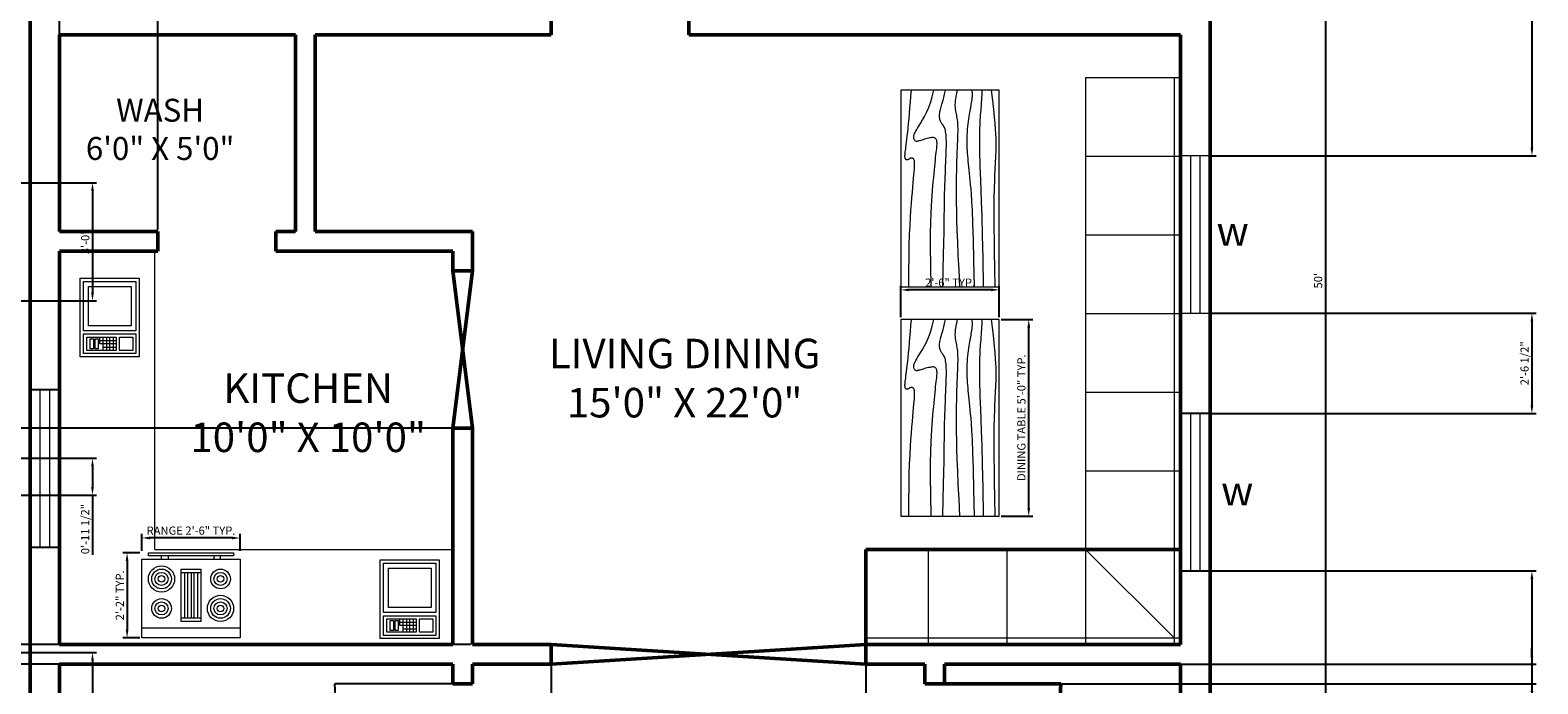
# Model space of a CAD drawing. Units: inches. Extents: x 3688 to 4628, y 1593 to 2337.
# Tile 6 of 7: x 4168 to 4628, y 1872 to 2072. Entities that reach past the tile are written whole.
import ezdxf

# ---------------------------------------------------------------- set-up
doc = ezdxf.new("R2010")
doc.units = ezdxf.units.IN
for name, color, linetype, lineweight in [('A-ANNO-DIMS', 2, 'Continuous', 18), ('A-ANNO-TEXT', 7, 'Continuous', 18), ('A-AREA-IDEN', 7, 'Continuous', 25), ('A-DOOR', 4, 'Continuous', 25), ('A-EQPM', 8, 'Continuous', 18), ('A-FLOR-FIXT', 8, 'Continuous', 18), ('A-FURN', 8, 'Continuous', 18), ('A-GLAZ', 4, 'Continuous', 25), ('A-WALL', 7, 'Continuous', 50)]:
    doc.layers.add(name, color=color, linetype=linetype, lineweight=lineweight)
doc.styles.get("Standard").update_dxf_attribs({"font": 'arial.ttf'})
doc.dimstyles.new('ISO-25', dxfattribs={"dimtxt": 2.5, "dimasz": 2.5, "dimexe": 1.25, "dimexo": 0.625, "dimtad": 1, "dimdec": 0, "dimlunit": 3, "dimtxsty": 'Standard', "dimcen": 2.5, "dimadec": 0, "dimazin": 0, "dimtfac": 1, "dimtdec": 0, "dimtmove": 0, "dimatfit": 3, "dimfxl": 1, "dimarcsym": 0})

# ---------------------------------------------------------------- blocks, each defined once
blk = doc.blocks.new('Microwave')
for p, q in [((18, 10), (22, 10)), ((19, 7), (19, 11)), ((20, 11), (20, 7)), ((21, 7), (21, 11)), ((22, 9), (18, 9)), ((18, 8), (22, 8)), ((22, 7), (18, 7)), ((20, 6), (18, 6)), ((19, 6), (19, 7)), ((20, 7), (20, 6))]:
    blk.add_line(p, q)
for points in [[(0, 0), (0, 18), (24, 18), (24, 0)], [(1, 1), (1, 17), (16, 17), (16, 1)], [(2.5, 2.5), (2.5, 15.5), (14.5, 15.5), (14.5, 2.5)], [(17, 1), (17, 17), (23, 17), (23, 1)], [(18, 12), (18, 16), (22, 16), (22, 12)], [(18, 2), (18, 11), (22, 11), (22, 2)], [(18.5, 4.5), (18.5, 5.5), (21.5, 5.5), (21.5, 4.5)], [(18.5, 3), (18.5, 4), (21.5, 4), (21.5, 3)]]:
    blk.add_lwpolyline(points, close=True)
blk = doc.blocks.new('Range-Oven - 30 in top')
for p, q in [((0, -3), (30, -3)), ((12, -6), (18, -6)), ((13, -20), (13, -6)), ((14, -6), (14, -20)), ((15, -20), (15, -6)), ((16, -6), (16, -20)), ((17, -20), (17, -6)), ((18, -20), (12, -20)), ((6, -24), (6, -25)), ((8, -25), (8, -24)), ((22, -25), (22, -24)), ((24, -24), (24, -25))]:
    blk.add_line(p, q)
for points in [[(0, -24), (0, 0), (30, 0), (30, -24)], [(12, -21), (12, -5), (18, -5), (18, -21)], [(2, -26), (2, -25), (28, -25), (28, -26)]]:
    blk.add_lwpolyline(points, close=True)
for centre, radius in [((6, -9), 4), ((6, -9), 3), ((6, -9), 2), ((6, -9), 1), ((24, -9), 3), ((24, -9), 2), ((24, -9), 1), ((6, -18), 3), ((6, -18), 2), ((6, -18), 1), ((24, -18), 4), ((24, -18), 3), ((24, -18), 2), ((24, -18), 1)]:
    blk.add_circle(centre, radius)
blk = doc.blocks.new('Table - Rectangular Woodgrain 60 x 30 in.')
for p, q in [((0, 0), (0, -30)), ((60, 0), (0, 0)), ((60, -30), (60, 0)), ((0, -30), (60, -30))]:
    blk.add_line(p, q)
for points in [[(0, -2.4), (4.8155, -2.418), (9.0302, -2.4688), (12.709, -2.5477), (15.9167, -2.65), (18.7181, -2.7711), (21.1781, -2.9063), (23.3616, -3.0508), (25.3333, -3.2), (27.1477, -3.3495), (28.8172, -3.4958), (30.3437, -3.636), (31.7291, -3.7667), (32.9756, -3.8849), (34.0849, -3.9875), (35.059, -4.0714), (35.9, -4.1334), (36.6114, -4.1711), (37.2041, -4.1854), (37.6906, -4.1779), (38.0833, -4.15), (38.3948, -4.1034), (38.6375, -4.0396), (38.8239, -3.9602), (38.9666, -3.8667), (39.0764, -3.7608), (39.1573, -3.6448), (39.2116, -3.521), (39.2416, -3.3917), (39.2498, -3.2593), (39.2385, -3.1261), (39.21, -2.9944), (39.1666, -2.8667), (39.111, -2.7447), (39.0468, -2.6281), (38.978, -2.5163), (38.9083, -2.4083), (38.8418, -2.3035), (38.7823, -2.201), (38.7337, -2.1001), (38.7, -2), (38.6844, -1.9003), (38.6875, -1.8021), (38.7094, -1.707), (38.75, -1.6167), (38.8094, -1.5326), (38.8875, -1.4563), (38.9844, -1.3893), (39.1, -1.3333), (39.2351, -1.2896), (39.3937, -1.2583), (39.5804, -1.2396), (39.8, -1.2333), (40.057, -1.2396), (40.3562, -1.2583), (40.7023, -1.2896), (41.1, -1.3333), (41.5547, -1.3895), (42.0755, -1.4573), (42.6721, -1.5361), (43.3542, -1.625), (44.1316, -1.7233), (45.014, -1.8302), (46.0114, -1.9449), (47.1333, -2.0667), (48.3862, -2.1947), (49.7625, -2.3281), (51.2513, -2.4663), (52.8416, -2.6083), (54.5226, -2.7535), (56.2833, -2.9011), (58.1127, -3.0501), (60, -3.2)], [(0, -9.2), (6.5759, -9.0858), (11.9385, -9.0365), (16.2527, -9.0418), (19.6833, -9.0917), (22.3952, -9.1759), (24.5531, -9.2844), (26.322, -9.4069), (27.8666, -9.5333), (29.3241, -9.6553), (30.7203, -9.7719), (32.0532, -9.8837), (33.3208, -9.9917), (34.5213, -10.0965), (35.6526, -10.199), (36.7128, -10.2999), (37.7, -10.4), (38.6129, -10.4996), (39.4531, -10.5969), (40.223, -10.6895), (40.925, -10.775), (41.5613, -10.8512), (42.1344, -10.9156), (42.6465, -10.966), (43.1, -11), (43.4976, -11.0158), (43.8437, -11.0136), (44.143, -10.9942), (44.4, -10.9583), (44.6195, -10.9069), (44.8062, -10.8406), (44.9648, -10.7603), (45.1, -10.6667), (45.2155, -10.5598), (45.3114, -10.4365), (45.3871, -10.2929), (45.4416, -10.125), (45.4743, -9.929), (45.4844, -9.7011), (45.4709, -9.4371), (45.4333, -9.1333), (45.3716, -8.7883), (45.2896, -8.4104), (45.1919, -8.0107), (45.0833, -7.6), (44.9685, -7.1893), (44.8521, -6.7896), (44.7388, -6.4117), (44.6333, -6.0667), (44.54, -5.7628), (44.4614, -5.4979), (44.4001, -5.2675), (44.3583, -5.0667), (44.3384, -4.8909), (44.3427, -4.7354), (44.3736, -4.5956), (44.4333, -4.4667), (44.5236, -4.3453), (44.6427, -4.2333), (44.7884, -4.1339), (44.9583, -4.05), (45.1501, -3.9849), (45.3614, -3.9417), (45.59, -3.9234), (45.8333, -3.9333), (46.0915, -3.9749), (46.3734, -4.0531), (46.6906, -4.1736), (47.0542, -4.3417), (47.4756, -4.5629), (47.9661, -4.8427), (48.5372, -5.1866), (49.2, -5.6), (49.9676, -6.0844), (50.8594, -6.625), (51.8965, -7.2031), (53.1, -7.8), (54.491, -8.3969), (56.0906, -8.975), (57.9199, -9.5156), (60, -10)], [(0, -12.8), (5.1847, -12.9322), (9.6213, -13.0323), (13.3963, -13.1059), (16.5958, -13.1583), (19.3063, -13.1952), (21.614, -13.2219), (23.6054, -13.2439), (25.3666, -13.2667), (26.9728, -13.2947), (28.4531, -13.3281), (29.8256, -13.3663), (31.1083, -13.4083), (32.3191, -13.4535), (33.476, -13.501), (34.597, -13.5501), (35.7, -13.6), (36.7984, -13.6497), (37.8875, -13.6979), (38.9578, -13.743), (40, -13.7833), (41.0047, -13.8174), (41.9625, -13.8438), (42.864, -13.8607), (43.7, -13.8667), (44.4631, -13.8604), (45.1552, -13.8417), (45.7801, -13.8104), (46.3416, -13.7667), (46.8439, -13.7104), (47.2906, -13.6417), (47.6858, -13.5604), (48.0333, -13.4667), (48.3375, -13.3608), (48.6042, -13.2448), (48.8396, -13.121), (49.05, -12.9917), (49.2417, -12.8593), (49.4208, -12.7261), (49.5937, -12.5944), (49.7667, -12.4667), (49.9452, -12.3451), (50.1323, -12.2313), (50.3303, -12.1268), (50.5416, -12.0333), (50.7686, -11.9524), (51.0135, -11.8854), (51.2788, -11.8341), (51.5666, -11.8), (51.8785, -11.7843), (52.2116, -11.7865), (52.562, -11.8059), (52.926, -11.8417), (53.2998, -11.8931), (53.6795, -11.9594), (54.0614, -12.0397), (54.4416, -12.1333), (54.8223, -12.2401), (55.2293, -12.3625), (55.6942, -12.5037), (56.2489, -12.6667), (56.9251, -12.8547), (57.7545, -13.0708), (58.7689, -13.3182), (60, -13.6)], [(0, -18), (5.124, -17.7273), (9.6609, -17.5057), (13.6705, -17.3303), (17.2125, -17.1958), (20.3467, -17.0973), (23.1328, -17.0297), (25.6307, -16.9878), (27.9, -16.9667), (29.9928, -16.9617), (31.9302, -16.9703), (33.7254, -16.9907), (35.3917, -17.0208), (36.9423, -17.0588), (38.3906, -17.1026), (39.7499, -17.1503), (41.0333, -17.2), (42.2519, -17.2496), (43.4073, -17.2969), (44.4986, -17.3395), (45.525, -17.375), (46.4858, -17.4012), (47.3802, -17.4156), (48.2074, -17.416), (48.9667, -17.4), (49.6583, -17.3662), (50.2872, -17.3167), (50.8595, -17.2547), (51.3812, -17.1833), (51.8584, -17.1057), (52.2971, -17.025), (52.7034, -16.9443), (53.0833, -16.8667), (53.443, -16.7951), (53.789, -16.7313), (54.128, -16.6768), (54.4666, -16.6334), (54.8115, -16.6024), (55.1693, -16.5854), (55.5465, -16.5841), (55.95, -16.6), (56.3828, -16.6337), (56.8346, -16.6823), (57.2915, -16.7418), (57.7396, -16.8084), (58.165, -16.878), (58.5539, -16.9469), (58.8924, -17.0111), (59.1666, -17.0667), (59.3679, -17.1107), (59.5078, -17.1438), (59.6032, -17.1675), (59.6708, -17.1833), (59.7275, -17.193), (59.7901, -17.1979), (59.8753, -17.1998), (60, -17.2)], [(0, -22.4), (8.0098, -22.2501), (14.4094, -22.1011), (19.4168, -21.9535), (23.25, -21.8083), (26.1269, -21.6663), (28.2656, -21.5281), (29.884, -21.3947), (31.2, -21.2667), (32.3967, -21.1448), (33.5172, -21.0292), (34.5697, -20.9198), (35.5625, -20.8167), (36.5037, -20.7198), (37.4015, -20.6292), (38.2642, -20.5448), (39.1, -20.4667), (39.9164, -20.3951), (40.7187, -20.3313), (41.5117, -20.2768), (42.3, -20.2333), (43.0883, -20.2024), (43.8812, -20.1854), (44.6836, -20.1841), (45.5, -20.2), (46.3328, -20.234), (47.1747, -20.2844), (48.0163, -20.3488), (48.8479, -20.425), (49.66, -20.5106), (50.4429, -20.6031), (51.1872, -20.7004), (51.8833, -20.8), (52.5246, -20.8999), (53.1166, -20.9995), (53.6681, -21.0983), (54.1875, -21.1958), (54.6834, -21.2919), (55.1646, -21.3859), (55.6394, -21.4777), (56.1167, -21.5667), (56.6028, -21.6515), (57.0961, -21.7266), (57.5929, -21.7852), (58.0896, -21.8208), (58.5823, -21.8268), (59.0674, -21.7964), (59.5412, -21.723), (60, -21.6)], [(0, -25.2), (8.6355, -25.0504), (15.7026, -24.9031), (21.4049, -24.7606), (25.9458, -24.625), (29.529, -24.4988), (32.3578, -24.3844), (34.6359, -24.284), (36.5667, -24.2), (38.3213, -24.1341), (39.9417, -24.0854), (41.437, -24.0523), (42.8167, -24.0333), (44.0901, -24.0268), (45.2667, -24.0313), (46.3557, -24.0451), (47.3667, -24.0667), (48.309, -24.0947), (49.1928, -24.1287), (50.0284, -24.168), (50.826, -24.2125), (51.5959, -24.2617), (52.3483, -24.3151), (53.0935, -24.3725), (53.8417, -24.4334), (54.6009, -24.497), (55.3699, -24.561), (56.1454, -24.6226), (56.9239, -24.6792), (57.7021, -24.7279), (58.4764, -24.7662), (59.2435, -24.7911), (60, -24.8)], [(0, -28.8), (5.6867, -28.6681), (10.45, -28.5698), (14.407, -28.5012), (17.675, -28.4584), (20.3711, -28.4374), (22.6125, -28.4344), (24.5164, -28.4455), (26.2, -28.4667), (27.762, -28.4947), (29.2276, -28.5281), (30.6033, -28.5663), (31.8958, -28.6084), (33.1118, -28.6535), (34.2578, -28.7011), (35.3405, -28.7501), (36.3666, -28.8), (37.3443, -28.8497), (38.288, -28.8974), (39.2137, -28.9412), (40.1375, -28.9792), (41.0753, -29.0093), (42.0432, -29.0297), (43.0572, -29.0384), (44.1333, -29.0333), (45.2936, -29.0114), (46.5843, -28.9641), (48.0579, -28.8816), (49.7666, -28.7542), (51.7629, -28.5721), (54.0989, -28.3255), (56.8272, -28.0048), (60, -27.6)]]:
    blk.add_lwpolyline(points)
blk = doc.blocks.new('*D15')
at = {"layer": 'A-ANNO-DIMS', "color": 0, "lineweight": -2, "transparency": 16777216}
for p, q in [((4528.76, 2295.28), (4564.58, 2295.28)), ((4563.33, 2292.78), (4563.33, 1697.78)), ((4528.76, 1695.28), (4564.58, 1695.28))]:
    blk.add_line(p, q, dxfattribs=at)
at = {"layer": 'A-ANNO-DIMS', "color": 0, "transparency": 16777216}
for points in [[(4562.91, 2292.78), (4563.75, 2292.78), (4563.33, 2295.28)], [(4562.91, 1697.78), (4563.75, 1697.78), (4563.33, 1695.28)]]:
    blk.add_solid(points, dxfattribs=at)
at = {"layer": 'Defpoints', "color": 0, "transparency": 16777216}
for p in [(4528.13, 2295.28), (4528.13, 1695.28), (4563.33, 1695.28)]:
    blk.add_point(p, dxfattribs=at)
at = {"layer": 'A-ANNO-DIMS', "color": 0, "transparency": 16777216, "insert": (4561.43, 1995.28), "char_height": 2.5, "attachment_point": 5, "rotation": 90}
blk.add_mtext("50'", dxfattribs=at)
blk = doc.blocks.new('DOOR-900')
blk.add_line((0, 0), (0, 36))
blk.add_arc((0, 0), 36, 0, 90)
blk = doc.blocks.new('WIN-1200')
for p, q in [((0, 48), (0, 0)), ((9, 48), (0, 48)), ((9, 0), (9, 48)), ((0, 0), (9, 0))]:
    blk.add_line(p, q)
blk = doc.blocks.new('*D41')
at = {"layer": 'A-ANNO-DIMS', "color": 0, "lineweight": -2, "transparency": 16777216}
for p, q in [((4464.44, 1983.48), (4474.06, 1983.48)), ((4472.81, 1925.98), (4472.81, 1980.98)), ((4464.44, 1923.48), (4474.06, 1923.48))]:
    blk.add_line(p, q, dxfattribs=at)
at = {"layer": 'A-ANNO-DIMS', "color": 0, "transparency": 16777216}
for points in [[(4472.39, 1980.98), (4473.23, 1980.98), (4472.81, 1983.48)], [(4472.39, 1925.98), (4473.23, 1925.98), (4472.81, 1923.48)]]:
    blk.add_solid(points, dxfattribs=at)
at = {"layer": 'Defpoints', "color": 0, "transparency": 16777216}
for p in [(4463.81, 1983.48), (4472.81, 1983.48), (4463.81, 1923.48)]:
    blk.add_point(p, dxfattribs=at)
at = {"layer": 'A-ANNO-DIMS', "color": 0, "transparency": 16777216, "insert": (4470.89, 1953.48), "char_height": 2.5, "attachment_point": 5, "rotation": 90}
blk.add_mtext('DINING TABLE 5\'-0" TYP.', dxfattribs=at)
blk = doc.blocks.new('*D42')
at = {"layer": 'A-ANNO-DIMS', "color": 0, "lineweight": -2, "transparency": 16777216}
for p, q in [((4433.81, 1984.11), (4433.81, 1993.73)), ((4461.31, 1992.48), (4436.31, 1992.48)), ((4463.81, 1984.11), (4463.81, 1993.73))]:
    blk.add_line(p, q, dxfattribs=at)
at = {"layer": 'A-ANNO-DIMS', "color": 0, "transparency": 16777216}
for points in [[(4436.31, 1992.9), (4436.31, 1992.07), (4433.81, 1992.48)], [(4461.31, 1992.9), (4461.31, 1992.07), (4463.81, 1992.48)]]:
    blk.add_solid(points, dxfattribs=at)
at = {"layer": 'Defpoints', "color": 0, "transparency": 16777216}
for p in [(4433.81, 1992.48), (4433.81, 1983.48), (4463.81, 1983.48)]:
    blk.add_point(p, dxfattribs=at)
at = {"layer": 'A-ANNO-DIMS', "color": 0, "transparency": 16777216, "insert": (4448.81, 1994.38), "char_height": 2.5, "attachment_point": 5}
blk.add_mtext('2\'-6" TYP.', dxfattribs=at)
blk = doc.blocks.new('*D45')
at = {"layer": 'A-ANNO-DIMS', "color": 0, "lineweight": -2, "transparency": 16777216}
for p, q in [((4202.21, 1912.91), (4202.21, 1918.04)), ((4229.71, 1916.79), (4204.71, 1916.79)), ((4232.21, 1912.91), (4232.21, 1918.04))]:
    blk.add_line(p, q, dxfattribs=at)
at = {"layer": 'A-ANNO-DIMS', "color": 0, "transparency": 16777216}
for points in [[(4204.71, 1917.21), (4204.71, 1916.37), (4202.21, 1916.79)], [(4229.71, 1917.21), (4229.71, 1916.37), (4232.21, 1916.79)]]:
    blk.add_solid(points, dxfattribs=at)
at = {"layer": 'Defpoints', "color": 0, "transparency": 16777216}
for p in [(4202.21, 1916.79), (4202.21, 1912.29), (4232.21, 1912.29)]:
    blk.add_point(p, dxfattribs=at)
at = {"layer": 'A-ANNO-DIMS', "color": 0, "transparency": 16777216, "insert": (4217.21, 1918.71), "char_height": 2.5, "attachment_point": 5}
blk.add_mtext('RANGE 2\'-6" TYP.', dxfattribs=at)
blk = doc.blocks.new('*D46')
at = {"layer": 'A-ANNO-DIMS', "color": 0, "lineweight": -2, "transparency": 16777216}
for p, q in [((4201.58, 1912.29), (4196.46, 1912.29)), ((4197.71, 1909.79), (4197.71, 1888.79)), ((4201.58, 1886.29), (4196.46, 1886.29))]:
    blk.add_line(p, q, dxfattribs=at)
at = {"layer": 'A-ANNO-DIMS', "color": 0, "transparency": 16777216}
for points in [[(4197.29, 1909.79), (4198.12, 1909.79), (4197.71, 1912.29)], [(4197.29, 1888.79), (4198.12, 1888.79), (4197.71, 1886.29)]]:
    blk.add_solid(points, dxfattribs=at)
at = {"layer": 'Defpoints', "color": 0, "transparency": 16777216}
for p in [(4202.21, 1912.29), (4197.71, 1886.29), (4202.21, 1886.29)]:
    blk.add_point(p, dxfattribs=at)
at = {"layer": 'A-ANNO-DIMS', "color": 0, "transparency": 16777216, "insert": (4195.82, 1899.29), "char_height": 2.5, "attachment_point": 5, "rotation": 90}
blk.add_mtext('2\'-2" TYP.', dxfattribs=at)
blk = doc.blocks.new('*D59')
at = {"layer": 'A-ANNO-DIMS', "color": 0, "lineweight": -2, "transparency": 16777216}
for p, q in [((4090.25, 2025.17), (4188.4, 2025.17)), ((4187.15, 2022.67), (4187.15, 1991.6)), ((4090.25, 1989.1), (4188.4, 1989.1))]:
    blk.add_line(p, q, dxfattribs=at)
at = {"layer": 'A-ANNO-DIMS', "color": 0, "transparency": 16777216}
for points in [[(4186.74, 2022.67), (4187.57, 2022.67), (4187.15, 2025.17)], [(4186.74, 1991.6), (4187.57, 1991.6), (4187.15, 1989.1)]]:
    blk.add_solid(points, dxfattribs=at)
at = {"layer": 'Defpoints', "color": 0, "transparency": 16777216}
for p in [(4089.62, 2025.17), (4089.62, 1989.1), (4187.15, 1989.1)]:
    blk.add_point(p, dxfattribs=at)
at = {"layer": 'A-ANNO-DIMS', "color": 0, "transparency": 16777216, "insert": (4185.25, 2007.14), "char_height": 2.5, "attachment_point": 5, "rotation": 90}
blk.add_mtext('3\'-0"', dxfattribs=at)
blk = doc.blocks.new('*D60')
at = {"layer": 'A-ANNO-DIMS', "color": 0, "lineweight": -2, "transparency": 16777216}
for p, q in [((4090.25, 1941.1), (4188.4, 1941.1)), ((4187.15, 1938.6), (4187.15, 1932.34)), ((4090.25, 1929.84), (4188.4, 1929.84)), ((4187.15, 1929.84), (4187.15, 1911.67))]:
    blk.add_line(p, q, dxfattribs=at)
at = {"layer": 'A-ANNO-DIMS', "color": 0, "transparency": 16777216}
for points in [[(4186.74, 1938.6), (4187.57, 1938.6), (4187.15, 1941.1)], [(4186.74, 1932.34), (4187.57, 1932.34), (4187.15, 1929.84)]]:
    blk.add_solid(points, dxfattribs=at)
at = {"layer": 'Defpoints', "color": 0, "transparency": 16777216}
for p in [(4089.62, 1941.1), (4089.62, 1929.84), (4187.15, 1929.84)]:
    blk.add_point(p, dxfattribs=at)
at = {"layer": 'A-ANNO-DIMS', "color": 0, "transparency": 16777216, "insert": (4185.24, 1919.5), "char_height": 2.5, "attachment_point": 5, "rotation": 90}
blk.add_mtext('0\'-11 1/2"', dxfattribs=at)
blk = doc.blocks.new('*D61')
at = {"layer": 'A-ANNO-DIMS', "color": 0, "lineweight": -2, "transparency": 16777216}
for p, q in [((4090.25, 1881.84), (4188.4, 1881.84)), ((4187.15, 1879.34), (4187.15, 1698.33)), ((4090.03, 1695.83), (4188.4, 1695.83))]:
    blk.add_line(p, q, dxfattribs=at)
at = {"layer": 'A-ANNO-DIMS', "color": 0, "transparency": 16777216}
for points in [[(4186.74, 1879.34), (4187.57, 1879.34), (4187.15, 1881.84)], [(4186.74, 1698.33), (4187.57, 1698.33), (4187.15, 1695.83)]]:
    blk.add_solid(points, dxfattribs=at)
at = {"layer": 'Defpoints', "color": 0, "transparency": 16777216}
for p in [(4089.62, 1881.84), (4089.41, 1695.83), (4187.15, 1695.83)]:
    blk.add_point(p, dxfattribs=at)
at = {"layer": 'A-ANNO-DIMS', "color": 0, "transparency": 16777216, "insert": (4185.25, 1788.83), "char_height": 2.5, "attachment_point": 5, "rotation": 90}
blk.add_mtext('15\'-6"', dxfattribs=at)
blk = doc.blocks.new('*D86')
at = {"layer": 'A-ANNO-DIMS', "color": 0, "lineweight": -2, "transparency": 16777216}
for p, q in [((4528.76, 2140.26), (4627.58, 2140.26)), ((4626.33, 2137.76), (4626.33, 2035.89)), ((4528.76, 2033.39), (4627.58, 2033.39))]:
    blk.add_line(p, q, dxfattribs=at)
at = {"layer": 'A-ANNO-DIMS', "color": 0, "transparency": 16777216}
for points in [[(4625.91, 2137.76), (4626.74, 2137.76), (4626.33, 2140.26)], [(4625.91, 2035.89), (4626.74, 2035.89), (4626.33, 2033.39)]]:
    blk.add_solid(points, dxfattribs=at)
at = {"layer": 'Defpoints', "color": 0, "transparency": 16777216}
for p in [(4528.13, 2140.26), (4528.13, 2033.39), (4626.33, 2033.39)]:
    blk.add_point(p, dxfattribs=at)
at = {"layer": 'A-ANNO-DIMS', "color": 0, "transparency": 16777216, "insert": (4624.43, 2086.83), "char_height": 2.5, "attachment_point": 5, "rotation": 90}
blk.add_mtext('8\'-11"', dxfattribs=at)
blk = doc.blocks.new('*D87')
at = {"layer": 'A-ANNO-DIMS', "color": 0, "lineweight": -2, "transparency": 16777216}
for p, q in [((4528.76, 1985.39), (4627.58, 1985.39)), ((4626.33, 1982.89), (4626.33, 1957.29)), ((4528.76, 1954.79), (4627.58, 1954.79))]:
    blk.add_line(p, q, dxfattribs=at)
at = {"layer": 'A-ANNO-DIMS', "color": 0, "transparency": 16777216}
for points in [[(4625.91, 1982.89), (4626.74, 1982.89), (4626.33, 1985.39)], [(4625.91, 1957.29), (4626.74, 1957.29), (4626.33, 1954.79)]]:
    blk.add_solid(points, dxfattribs=at)
at = {"layer": 'Defpoints', "color": 0, "transparency": 16777216}
for p in [(4528.13, 1985.39), (4528.13, 1954.79), (4626.33, 1954.79)]:
    blk.add_point(p, dxfattribs=at)
at = {"layer": 'A-ANNO-DIMS', "color": 0, "transparency": 16777216, "insert": (4624.41, 1970.09), "char_height": 2.5, "attachment_point": 5, "rotation": 90}
blk.add_mtext('2\'-6 1/2"', dxfattribs=at)
blk = doc.blocks.new('*D88')
at = {"layer": 'A-ANNO-DIMS', "color": 0, "lineweight": -2, "transparency": 16777216}
for p, q in [((4528.76, 1906.79), (4627.58, 1906.79)), ((4626.33, 1904.29), (4626.33, 1697.78)), ((4528.76, 1695.28), (4627.58, 1695.28))]:
    blk.add_line(p, q, dxfattribs=at)
at = {"layer": 'A-ANNO-DIMS', "color": 0, "transparency": 16777216}
for points in [[(4625.91, 1904.29), (4626.74, 1904.29), (4626.33, 1906.79)], [(4625.91, 1697.78), (4626.74, 1697.78), (4626.33, 1695.28)]]:
    blk.add_solid(points, dxfattribs=at)
at = {"layer": 'Defpoints', "color": 0, "transparency": 16777216}
for p in [(4528.13, 1906.79), (4528.13, 1695.28), (4626.33, 1695.28)]:
    blk.add_point(p, dxfattribs=at)
at = {"layer": 'A-ANNO-DIMS', "color": 0, "transparency": 16777216, "insert": (4624.41, 1801.03), "char_height": 2.5, "attachment_point": 5, "rotation": 90}
blk.add_mtext('17\'-7 1/2"', dxfattribs=at)
blk = doc.blocks.new('*D98')
at = {"layer": 'A-ANNO-DIMS', "color": 0, "lineweight": -2, "transparency": 16777216}
for p, q in [((4177.13, 2010.91), (4177.13, 2332.13)), ((4179.63, 2330.88), (4204.63, 2330.88)), ((4207.13, 2010.91), (4207.13, 2332.13))]:
    blk.add_line(p, q, dxfattribs=at)
at = {"layer": 'A-ANNO-DIMS', "color": 0, "transparency": 16777216}
for points in [[(4179.63, 2331.3), (4179.63, 2330.47), (4177.13, 2330.88)], [(4204.63, 2331.3), (4204.63, 2330.47), (4207.13, 2330.88)]]:
    blk.add_solid(points, dxfattribs=at)
at = {"layer": 'Defpoints', "color": 0, "transparency": 16777216}
for p in [(4207.13, 2330.88), (4177.13, 2010.28), (4207.13, 2010.28)]:
    blk.add_point(p, dxfattribs=at)
at = {"layer": 'A-ANNO-DIMS', "color": 0, "transparency": 16777216, "insert": (4192.13, 2332.78), "char_height": 2.5, "attachment_point": 5}
blk.add_mtext('2\'-6"', dxfattribs=at)
blk = doc.blocks.new('*D99')
at = {"layer": 'A-ANNO-DIMS', "color": 0, "lineweight": -2, "transparency": 16777216}
for p, q in [((4302.51, 1950.28), (4055.24, 1950.28)), ((4056.49, 1947.78), (4056.49, 1886.78)), ((4302.51, 1884.28), (4055.24, 1884.28))]:
    blk.add_line(p, q, dxfattribs=at)
at = {"layer": 'A-ANNO-DIMS', "color": 0, "transparency": 16777216}
for points in [[(4056.07, 1947.78), (4056.9, 1947.78), (4056.49, 1950.28)], [(4056.07, 1886.78), (4056.9, 1886.78), (4056.49, 1884.28)]]:
    blk.add_solid(points, dxfattribs=at)
at = {"layer": 'Defpoints', "color": 0, "transparency": 16777216}
for p in [(4303.13, 1950.28), (4056.49, 1884.28), (4303.13, 1884.28)]:
    blk.add_point(p, dxfattribs=at)
at = {"layer": 'A-ANNO-DIMS', "color": 0, "transparency": 16777216, "insert": (4054.58, 1917.28), "char_height": 2.5, "attachment_point": 5, "rotation": 90}
blk.add_mtext('5\'-6"', dxfattribs=at)
blk = doc.blocks.new('*D100')
at = {"layer": 'A-ANNO-DIMS', "color": 0, "lineweight": -2, "transparency": 16777216}
for p, q in [((4327.13, 1883.66), (4327.13, 1595.79)), ((4423.13, 1883.66), (4423.13, 1595.79)), ((4329.63, 1597.04), (4420.63, 1597.04))]:
    blk.add_line(p, q, dxfattribs=at)
at = {"layer": 'A-ANNO-DIMS', "color": 0, "transparency": 16777216}
for points in [[(4329.63, 1597.45), (4329.63, 1596.62), (4327.13, 1597.04)], [(4420.63, 1597.45), (4420.63, 1596.62), (4423.13, 1597.04)]]:
    blk.add_solid(points, dxfattribs=at)
at = {"layer": 'Defpoints', "color": 0, "transparency": 16777216}
for p in [(4327.13, 1884.28), (4423.13, 1884.28), (4423.13, 1597.04)]:
    blk.add_point(p, dxfattribs=at)
at = {"layer": 'A-ANNO-DIMS', "color": 0, "transparency": 16777216, "insert": (4375.13, 1598.94), "char_height": 2.5, "attachment_point": 5}
blk.add_mtext('8\'-0"', dxfattribs=at)
blk = doc.blocks.new('*D101')
at = {"layer": 'A-ANNO-DIMS', "color": 0, "lineweight": -2, "transparency": 16777216}
for p, q in [((4056.49, 1886.78), (4056.49, 1889.28)), ((4296.51, 1884.28), (4055.24, 1884.28)), ((4056.49, 1884.28), (4056.49, 1878.28)), ((4296.51, 1878.28), (4055.24, 1878.28)), ((4056.49, 1875.78), (4056.49, 1865.39))]:
    blk.add_line(p, q, dxfattribs=at)
at = {"layer": 'A-ANNO-DIMS', "color": 0, "transparency": 16777216}
for points in [[(4056.07, 1886.78), (4056.9, 1886.78), (4056.49, 1884.28)], [(4056.07, 1875.78), (4056.9, 1875.78), (4056.49, 1878.28)]]:
    blk.add_solid(points, dxfattribs=at)
at = {"layer": 'Defpoints', "color": 0, "transparency": 16777216}
for p in [(4297.13, 1884.28), (4056.49, 1878.28), (4297.13, 1878.28)]:
    blk.add_point(p, dxfattribs=at)
at = {"layer": 'A-ANNO-DIMS', "color": 0, "transparency": 16777216, "insert": (4054.58, 1869.34), "char_height": 2.5, "attachment_point": 5, "rotation": 90}
blk.add_mtext('0\'-6"', dxfattribs=at)
blk = doc.blocks.new('*D103')
at = {"layer": 'A-ANNO-DIMS', "color": 0, "lineweight": -2, "transparency": 16777216}
for p, q in [((4626.33, 1880.78), (4626.33, 1883.28)), ((4447.76, 1878.28), (4627.58, 1878.28)), ((4626.33, 1878.28), (4626.33, 1872.28)), ((4447.76, 1872.28), (4627.58, 1872.28)), ((4626.33, 1869.78), (4626.33, 1859.39))]:
    blk.add_line(p, q, dxfattribs=at)
at = {"layer": 'A-ANNO-DIMS', "color": 0, "transparency": 16777216}
for points in [[(4625.91, 1880.78), (4626.74, 1880.78), (4626.33, 1878.28)], [(4625.91, 1869.78), (4626.74, 1869.78), (4626.33, 1872.28)]]:
    blk.add_solid(points, dxfattribs=at)
at = {"layer": 'Defpoints', "color": 0, "transparency": 16777216}
for p in [(4447.13, 1878.28), (4447.13, 1872.28), (4626.33, 1872.28)]:
    blk.add_point(p, dxfattribs=at)
at = {"layer": 'A-ANNO-DIMS', "color": 0, "transparency": 16777216, "insert": (4624.43, 1863.34), "char_height": 2.5, "attachment_point": 5, "rotation": 90}
blk.add_mtext('0\'-6"', dxfattribs=at)

msp = doc.modelspace()

# ---------------------------------------------------------------- linework, layer by layer
at = {"layer": 'A-FLOR-FIXT'}
for p, q in [((4206.13, 1913.28), (4206.13, 2004.28)), ((4206.13, 1913.28), (4255.13, 1913.28)), ((4255.13, 1913.28), (4297.13, 1913.28))]:
    msp.add_line(p, q, dxfattribs=at)
at = {"layer": 'A-FURN'}
for p, q in [((4490.13, 2057.28), (4490.13, 1884.28)), ((4490.13, 2057.28), (4519.13, 2057.28)), ((4517.13, 2057.28), (4517.13, 1884.28)), ((4490.13, 2033.28), (4519.13, 2033.28)), ((4519.13, 2033.39), (4519.13, 1985.39)), ((4528.13, 2033.39), (4519.13, 2033.39)), ((4522.13, 2033.39), (4522.13, 1985.39)), ((4525.13, 1985.39), (4525.13, 2033.39)), ((4528.13, 1985.39), (4528.13, 2033.39)), ((4490.13, 2009.28), (4519.13, 2009.28)), ((4490.13, 1985.28), (4519.13, 1985.28)), ((4519.13, 1985.39), (4528.13, 1985.39)), ((4171.13, 1962.02), (4171.13, 1914.02)), ((4174.13, 1914.02), (4174.13, 1962.02)), ((4490.13, 1961.28), (4519.13, 1961.28)), ((4522.13, 1954.79), (4522.13, 1906.79)), ((4525.13, 1906.79), (4525.13, 1954.79)), ((4490.13, 1937.28), (4519.13, 1937.28)), ((4442.13, 1913.28), (4442.13, 1884.28)), ((4466.13, 1913.28), (4466.13, 1884.28)), ((4490.13, 1913.28), (4517.13, 1886.28)), ((4423.13, 1886.28), (4519.13, 1886.28))]:
    msp.add_line(p, q, dxfattribs=at)
at = {"layer": 'A-WALL'}
for p, q in [((4168.13, 1695.28), (4168.13, 2295.28)), ((4528.13, 2295.28), (4528.13, 1695.28)), ((4327.13, 2082.28), (4327.13, 2070.28)), ((4369.13, 2082.28), (4369.13, 2070.28)), ((4177.13, 2070.28), (4249.13, 2070.28)), ((4177.13, 2010.28), (4177.13, 2070.28)), ((4249.13, 2010.28), (4249.13, 2070.28)), ((4255.13, 2010.28), (4255.13, 2070.28)), ((4255.13, 2070.28), (4321.13, 2070.28)), ((4321.13, 2070.28), (4327.13, 2070.28)), ((4375.13, 2070.28), (4369.13, 2070.28)), ((4375.13, 2070.28), (4519.13, 2070.28)), ((4519.13, 2070.28), (4519.13, 1884.28)), ((4177.13, 2010.28), (4207.13, 2010.28)), ((4207.13, 2004.28), (4207.13, 2010.28)), ((4249.13, 2010.28), (4243.13, 2010.28)), ((4243.13, 2010.28), (4243.13, 2004.28)), ((4243.13, 2010.28), (4249.13, 2010.28)), ((4255.13, 2010.28), (4303.13, 2010.28)), ((4303.13, 1998.28), (4303.13, 2010.28)), ((4177.13, 2004.28), (4207.13, 2004.28)), ((4177.13, 1884.28), (4177.13, 2004.28)), ((4243.13, 2004.28), (4255.13, 2004.28)), ((4255.13, 2004.28), (4297.13, 2004.28)), ((4297.13, 2004.28), (4297.13, 1998.28)), ((4297.13, 1998.28), (4297.13, 2004.28)), ((4297.13, 1998.28), (4303.13, 1998.28)), ((4303.13, 1998.28), (4297.13, 1950.28)), ((4303.13, 1950.28), (4297.13, 1998.28)), ((4297.13, 1884.28), (4297.13, 1950.28)), ((4303.13, 1950.28), (4297.13, 1950.28)), ((4297.13, 1950.28), (4303.13, 1950.28)), ((4303.13, 1884.28), (4303.13, 1950.28)), ((4423.13, 1913.28), (4519.13, 1913.28)), ((4423.13, 1913.28), (4423.13, 1884.28)), ((4177.13, 1884.28), (4255.13, 1884.28)), ((4255.13, 1884.28), (4297.13, 1884.28)), ((4303.13, 1884.28), (4327.13, 1884.28)), ((4327.13, 1884.28), (4327.13, 1878.28)), ((4327.13, 1884.28), (4423.13, 1878.28)), ((4423.13, 1884.28), (4327.13, 1878.28)), ((4423.13, 1878.28), (4423.13, 1884.28)), ((4423.13, 1884.28), (4519.13, 1884.28)), ((4423.13, 1878.28), (4423.13, 1884.28)), ((4177.13, 1878.28), (4255.13, 1878.28)), ((4177.13, 1758.28), (4177.13, 1878.28)), ((4255.13, 1878.28), (4297.13, 1878.28)), ((4297.13, 1878.28), (4297.13, 1872.28)), ((4297.13, 1872.28), (4297.13, 1878.28)), ((4303.13, 1878.28), (4327.13, 1878.28)), ((4303.13, 1878.28), (4327.13, 1878.28)), ((4303.13, 1872.28), (4303.13, 1878.28)), ((4303.13, 1872.28), (4303.13, 1878.28)), ((4423.13, 1878.28), (4441.13, 1878.28)), ((4441.13, 1878.28), (4441.13, 1872.28)), ((4441.13, 1878.28), (4441.13, 1872.28)), ((4447.13, 1878.28), (4447.13, 1872.28)), ((4447.13, 1878.28), (4519.13, 1878.28)), ((4519.13, 1878.28), (4519.13, 1818.28)), ((4297.13, 1872.28), (4303.13, 1872.28)), ((4441.13, 1872.28), (4447.13, 1872.28)), ((4447.13, 1872.28), (4482.58, 1872.28))]:
    msp.add_line(p, q, dxfattribs=at)
msp.add_arc((4447.13, 1872.28), 35.44, 270, 0, dxfattribs=at)

# ---------------------------------------------------------------- block references
at = {"layer": 'A-DOOR', "extrusion": (0, 0, -1), "zscale": -1, "rotation": 270}
msp.add_blockref('DOOR-900', (-4297.13, 1872.28), dxfattribs=at)
at = {"layer": 'A-EQPM'}
for name, p, rotation in [('Microwave', (4183.42, 1996.03), 270), ('Range-Oven - 30 in top', (4232.21, 1886.29), 180), ('Microwave', (4274.95, 1910.08), 270)]:
    msp.add_blockref(name, p, dxfattribs=dict(at, rotation=rotation))
at = {"layer": 'A-FURN', "rotation": 90}
for p in [(4433.81, 1993.46), (4433.81, 1923.48)]:
    msp.add_blockref('Table - Rectangular Woodgrain 60 x 30 in.', p, dxfattribs=at)
at = {"layer": 'A-GLAZ'}
for p in [(4168.13, 1914.03), (4519.13, 1906.79)]:
    msp.add_blockref('WIN-1200', p, dxfattribs=at)

# ---------------------------------------------------------------- texts
at = {"layer": 'A-ANNO-TEXT', "char_height": 9, "attachment_point": 1}
for insert in [(4465.79, 2014.95), (4467.18, 1935.73)]:
    msp.add_mtext_dynamic_manual_height_columns('\\pxqc;w', width=138.4723, gutter_width=12.5, heights=[0], dxfattribs=dict(at, insert=insert))
at = {"layer": 'A-AREA-IDEN', "attachment_point": 1}
for s, width, insert, char_height in [('\\pxqc;WASH\\P6\'0" X 5\'0"', 61.3205, (4177.13, 2050.79), 7), ('\\pxqc;LIVING DINING\\P15\'0" X 22\'0"', 105.0766, (4315.28, 1977.57), 9), ('\\pxqc;KITCHEN^J10\'0" X 10\'0"', 105.0766, (4200.43, 1967.01), 9)]:
    msp.add_mtext_dynamic_manual_height_columns(s, width=width, gutter_width=12.5, heights=[0], dxfattribs=dict(at, insert=insert, char_height=char_height))

# ---------------------------------------------------------------- dimensions: what is measured, and where the dimension line sits
at = {"layer": 'A-ANNO-DIMS'}
for base, p1, p2, picture, middle in [((4207.13, 2330.88), (4177.13, 2010.28), (4207.13, 2010.28), '*D98', (4192.13, 2332.78)), ((4423.13, 1597.04), (4327.13, 1884.28), (4423.13, 1884.28), '*D100', (4375.13, 1598.94))]:
    dim = msp.add_linear_dim(base=base, p1=p1, p2=p2, dimstyle='ISO-25', override={"dimdec": 1, "dimlfac": 1, "dimrnd": 0, "dimzin": 1, "dimdsep": 46, "dimlunit": 4, "dimfrac": 2}, dxfattribs=at)
    dim.commit()
    dim.dimension.update_dxf_attribs({"geometry": picture, "text_midpoint": middle})
for base, p1, p2, override, picture, middle in [((4563.33, 1695.28), (4528.13, 2295.28), (4528.13, 1695.28), {"dimclrd": 0, "dimclre": 0, "dimclrt": 0}, '*D15', (4561.43, 1995.28)), ((4626.33, 2033.39), (4528.13, 2140.26), (4528.13, 2033.39), {"dimdec": 1, "dimlfac": 1, "dimrnd": 0, "dimzin": 1, "dimdsep": 46, "dimlunit": 4, "dimfrac": 2}, '*D86', (4624.43, 2086.83)), ((4187.15, 1989.1), (4089.62, 2025.17), (4089.62, 1989.1), {"dimdec": 1, "dimlfac": 1, "dimrnd": 0, "dimzin": 1, "dimdsep": 46, "dimlunit": 4, "dimfrac": 2}, '*D59', (4185.25, 2007.14)), ((4626.33, 1954.79), (4528.13, 1985.39), (4528.13, 1954.79), {"dimdec": 1, "dimlfac": 1, "dimrnd": 0, "dimzin": 1, "dimdsep": 46, "dimlunit": 4, "dimfrac": 2}, '*D87', (4624.41, 1970.09)), ((4056.49, 1884.28), (4303.13, 1950.28), (4303.13, 1884.28), {"dimdec": 1, "dimlfac": 1, "dimrnd": 0, "dimzin": 1, "dimdsep": 46, "dimlunit": 4, "dimfrac": 2}, '*D99', (4054.58, 1917.28)), ((4187.15, 1929.84), (4089.62, 1941.1), (4089.62, 1929.84), {"dimdec": 1, "dimlfac": 1, "dimrnd": 0, "dimzin": 1, "dimdsep": 46, "dimlunit": 4, "dimfrac": 2}, '*D60', (4185.24, 1919.5)), ((4626.33, 1695.28), (4528.13, 1906.79), (4528.13, 1695.28), {"dimdec": 1, "dimlfac": 1, "dimrnd": 0, "dimzin": 1, "dimdsep": 46, "dimlunit": 4, "dimfrac": 2}, '*D88', (4624.41, 1801.03)), ((4056.49, 1878.28), (4297.13, 1884.28), (4297.13, 1878.28), {"dimdec": 1, "dimlfac": 1, "dimrnd": 0, "dimzin": 1, "dimdsep": 46, "dimlunit": 4, "dimfrac": 2}, '*D101', (4054.58, 1869.34)), ((4187.15, 1695.83), (4089.62, 1881.84), (4089.41, 1695.83), {"dimdec": 1, "dimlfac": 1, "dimrnd": 0, "dimzin": 1, "dimdsep": 46, "dimlunit": 4, "dimfrac": 2}, '*D61', (4185.25, 1788.83)), ((4626.33, 1872.28), (4447.13, 1878.28), (4447.13, 1872.28), {"dimdec": 1, "dimlfac": 1, "dimrnd": 0, "dimzin": 1, "dimdsep": 46, "dimlunit": 4, "dimfrac": 2}, '*D103', (4624.43, 1863.34))]:
    dim = msp.add_linear_dim(base=base, p1=p1, p2=p2, angle=90, dimstyle='ISO-25', override=override, dxfattribs=at)
    dim.commit()
    dim.dimension.update_dxf_attribs({"geometry": picture, "text_midpoint": middle})
for base, p1, p2, angle, text, picture, middle in [((4433.81, 1992.48), (4463.81, 1983.48), (4433.81, 1983.48), 180, '<> TYP.', '*D42', (4448.81, 1994.38)), ((4472.81, 1983.48), (4463.81, 1923.48), (4463.81, 1983.48), 90, 'DINING TABLE <> TYP.', '*D41', (4470.89, 1953.48)), ((4202.21, 1916.79), (4232.21, 1912.29), (4202.21, 1912.29), 180, 'RANGE <> TYP.', '*D45', (4217.21, 1918.71)), ((4197.71, 1886.29), (4202.21, 1912.29), (4202.21, 1886.29), 270, '<> TYP.', '*D46', (4195.82, 1899.29))]:
    dim = msp.add_linear_dim(base=base, p1=p1, p2=p2, angle=angle, text=text, dimstyle='ISO-25', override={"dimdec": 1, "dimrnd": 0, "dimzin": 1, "dimlunit": 4, "dimfrac": 2}, dxfattribs=at)
    dim.commit()
    dim.dimension.update_dxf_attribs({"geometry": picture, "text_midpoint": middle})

doc.saveas('drawing.dxf')
